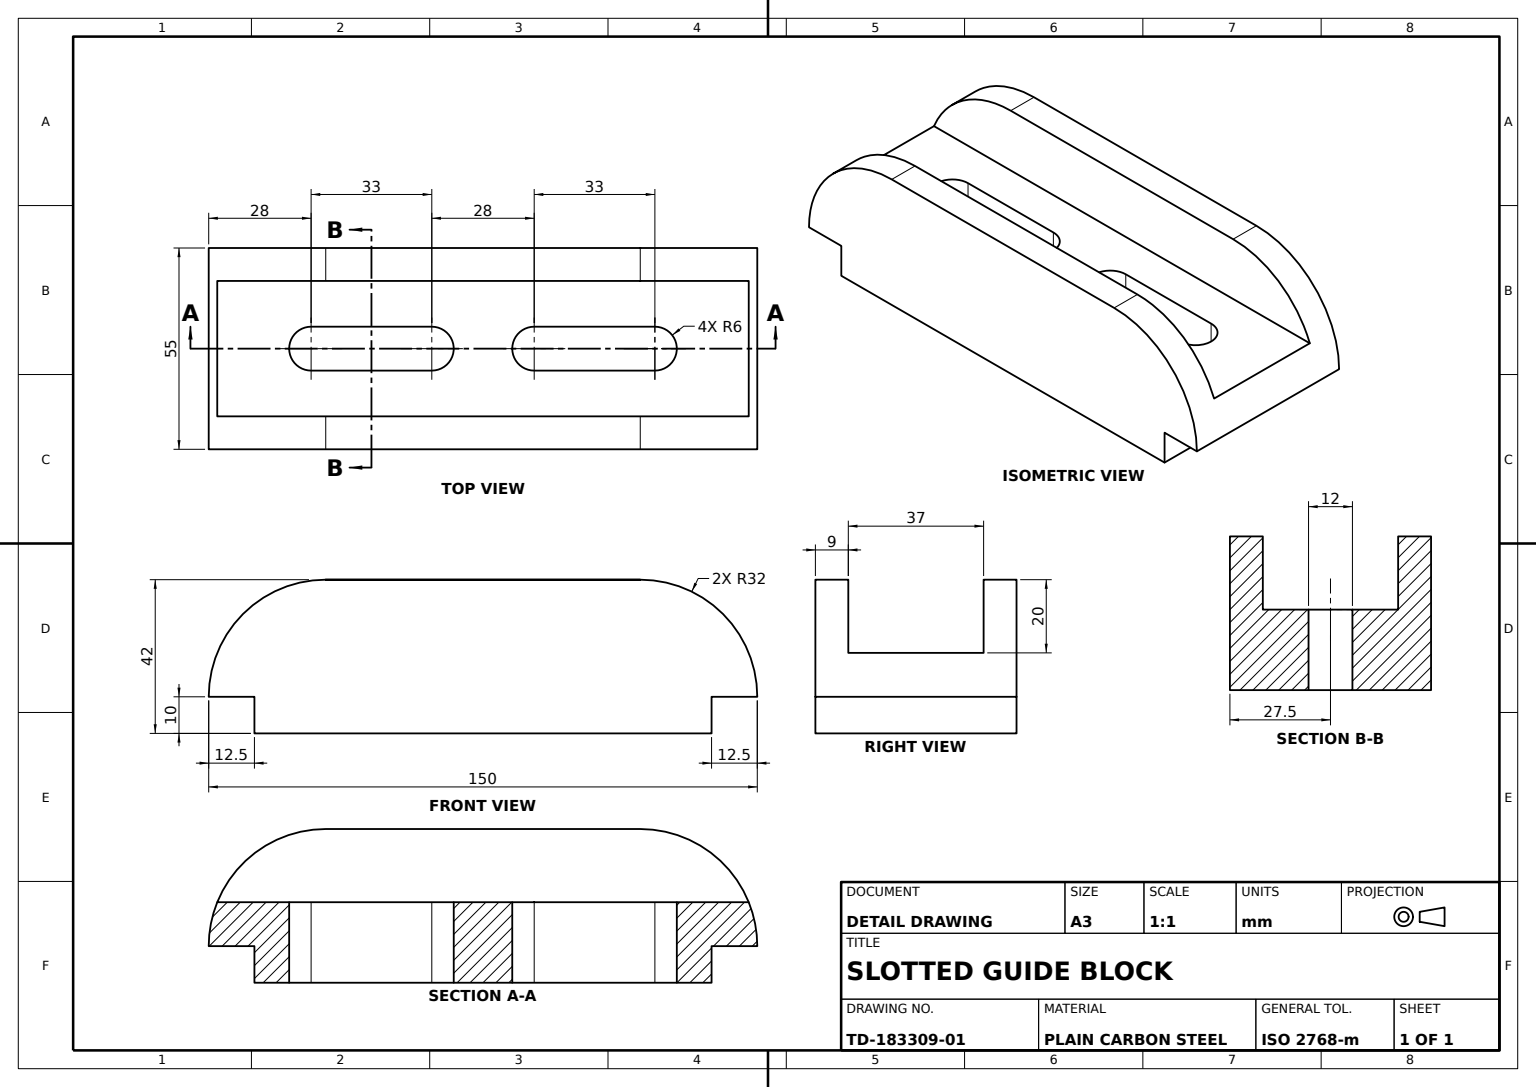
from build123d import *

# Parameters (mm, degrees)
SLIDE_BLOCK_BODY_DEPTH       = 27.5
CENTRE_CHANNEL_37_WIDE_DEPTH = 20
TWIN_SLOTS_2XR6_DEPTH        = 38


with BuildPart() as part:
    # Block Profile Sketch → Slide Block Body (new, symmetric)
    with BuildSketch(Plane.XY):
        with BuildLine():
            Line((0, 0), (62.5, 0))
            Line((62.5, 0), (62.5, 10))
            Line((62.5, 10), (75, 10))
            ThreePointArc((75, 10), (65.627416998, 32.627416998), (43, 42))
            Line((43, 42), (0, 42))
            Line((0, 42), (-43, 42))
            ThreePointArc((-43, 42), (-65.627416998, 32.627416998), (-75, 10))
            Line((-75, 10), (-62.5, 10))
            Line((-62.5, 10), (-62.5, 0))
            Line((-62.5, 0), (0, 0))
        make_face()
    extrude(amount=SLIDE_BLOCK_BODY_DEPTH, both=True)

    # Centre Channel Sketch → Centre Channel 37 Wide (cut)
    with BuildSketch(Plane(origin=(0, 42, 0), x_dir=(1, 0, 0), z_dir=(0, 1, 0))):
        Polygon((0, 18.5), (92.62343554, 18.5), (92.62343554, -18.5), (-101.990097212, -18.5), (-101.990097212, 18.5), align=None)
    extrude(amount=-CENTRE_CHANNEL_37_WIDE_DEPTH, mode=Mode.SUBTRACT)

    # Twin Slots Sketch → Twin Slots 2xR6 (cut)
    with BuildSketch(Plane(origin=(0, 22, 0), x_dir=(1, 0, 0), z_dir=(0, 1, 0))):
        with BuildLine():
            Line((-14, -6), (-47, -6))
            ThreePointArc((-47, -6), (-53, 0), (-47, 6))
            Line((-47, 6), (-14, 6))
            ThreePointArc((-14, 6), (-8, 0), (-14, -6))
        make_face()
        with BuildLine():
            Line((14, 6), (47, 6))
            ThreePointArc((47, 6), (53, 0), (47, -6))
            Line((47, -6), (14, -6))
            ThreePointArc((14, -6), (8, 0), (14, 6))
        make_face()
    extrude(amount=-TWIN_SLOTS_2XR6_DEPTH, mode=Mode.SUBTRACT)


solid = part.part
